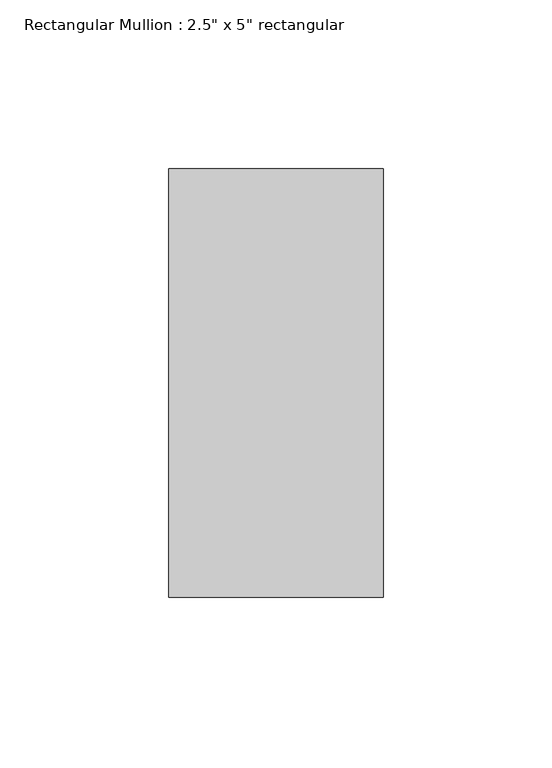
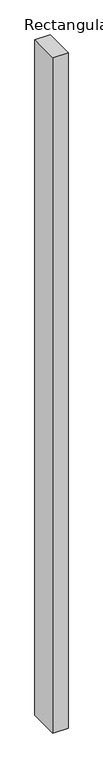
"""IFC4 building model written with IfcOpenShell, lengths in millimetres: member geometry."""

from ifc_helpers import new_model, si_unit, frame, origin, place, context, project, spatial, polyline, outline, extrude, source, transform, mapped, element, save


def member_daa7a266(model_context):
    return source(origin(), model_context, "Body", "SweptSolid", [
        extrude(outline(polyline([(0.0, 63.5), (0.0, -63.5), (-63.5, -63.5), (-63.5, 63.5), (0.0, 63.5)])), frame((0.0, 0.0, -2952.7500003), z_axis=(0.0, 0.0, 1.0), x_axis=(1.0, 0.0, 0.0)), (0.0, 0.0, 1.0), 2952.7500003),
    ])


if __name__ == "__main__":
    model = new_model("IFC4")
    model_context = context("Model", 3, world=origin())
    ifc_project = project(units=[si_unit("LENGTHUNIT", "METRE", prefix="MILLI")], contexts=[model_context])
    site = spatial("IfcSite", under=ifc_project)
    building = spatial("IfcBuilding", under=site)
    placement = place(None, origin())
    member_shape = member_daa7a266(model_context)
    element("IfcMember", 1, ObjectType="Rectangular Mullion : 2.5\" x 5\" rectangular", at=placement, inside=building, context=model_context, shape_type="MappedRepresentation", body=[
        mapped(member_shape, transform((0.0, 0.0, 0.0), x_axis=(1.0, 0.0, 0.0), y_axis=(0.0, 1.0, 0.0), z_axis=(0.0, 0.0, 1.0))),
    ])
    save(model, "model.ifc")

# Revit data of these elements
# Type "Rectangular Mullion : 2.5\" x 5\" rectangular"
#   built-in parameter 1007304 = 0.416667 (stored number, unit not read)
#   built-in parameter 1007301 = 0.104167 (stored number, unit not read)
#   built-in parameter 1007300 = 0.104167 (stored number, unit not read)
# Element 1 (IfcMember, "Rectangular Mullion : 2.5\" x 5\" rectangular")
#   Materials on its faces: "Aluminum"
# Materials
#   "Aluminum": class "Metal", colour RGB 247 247 247, transparency 0, Description = "Aluminum 6061", Cost = 0
